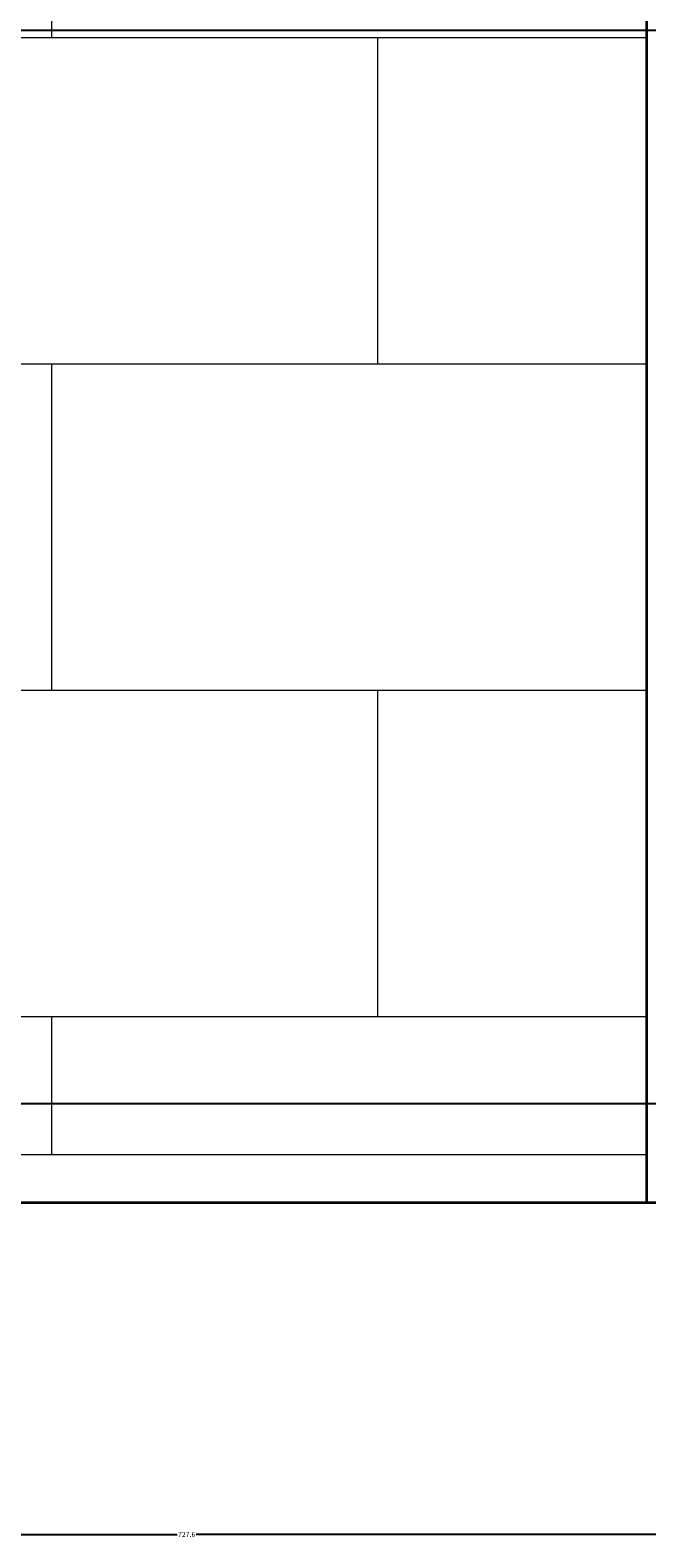
# Model space of a CAD drawing. Units: inches. Extents: x -26 to 776, y -22 to 650.
# Tile 17 of 62: x 358 to 426, y -22 to 145. Entities that reach past the tile are written whole.
import ezdxf

# ---------------------------------------------------------------- set-up
doc = ezdxf.new("R2010")
doc.units = ezdxf.units.IN
doc.header["$MEASUREMENT"] = 0
for name, color, linetype, lineweight in [('A-ANNO-DIMS', 2, 'Continuous', 18), ('A-WALL', 7, 'Continuous', 35), ('A-WALL-PATT', 8, 'Continuous', 13), ('A-WALL-TRIM', 7, 'Continuous', 18), ('C-TOPO', 7, 'Continuous', 35)]:
    doc.layers.add(name, color=color, linetype=linetype, lineweight=lineweight)
doc.styles.get("Standard").update_dxf_attribs({"font": 'arial.ttf'})
doc.dimstyles.get("Standard").update_dxf_attribs({"dimtxt": 0.5625, "dimasz": 0.18, "dimexe": 0.18, "dimexo": 0.0625, "dimgap": 0.09, "dimtad": 0, "dimtih": 1, "dimtoh": 1, "dimdec": 4, "dimzin": 0, "dimdsep": 46, "dimlunit": 4, "dimtxsty": 'Standard', "dimcen": 0.09, "dimadec": 0, "dimazin": 0, "dimtfac": 1, "dimtdec": 4, "dimtofl": 0, "dimtmove": 0, "dimatfit": 3, "dimfxl": 1, "dimtolj": 1, "dimtzin": 0, "dimarcsym": 0})

# ---------------------------------------------------------------- blocks, each defined once
blk = doc.blocks.new('*D13')
at = {"layer": 'A-ANNO-DIMS', "color": 0, "lineweight": -2, "transparency": 16777216}
for p, q in [((738.75, 50.79), (738.75, -21.31)), ((11.11, 15.42), (11.11, -21.31)), ((11.29, -21.13), (373.89, -21.13)), ((738.57, -21.13), (375.97, -21.13))]:
    blk.add_line(p, q, dxfattribs=at)
at = {"layer": 'A-ANNO-DIMS', "color": 0, "transparency": 16777216}
for points in [[(11.29, -21.1), (11.29, -21.16), (11.11, -21.13)], [(738.57, -21.1), (738.57, -21.16), (738.75, -21.13)]]:
    blk.add_solid(points, dxfattribs=at)
at = {"layer": 'Defpoints', "color": 0, "transparency": 16777216}
for p in [(738.75, 50.85), (11.11, 15.48), (738.75, -21.13)]:
    blk.add_point(p, dxfattribs=at)
at = {"layer": 'A-ANNO-DIMS', "color": 0, "transparency": 16777216, "insert": (374.93, -21.13), "char_height": 0.562, "attachment_point": 5}
blk.add_mtext('\\A1;727.6', dxfattribs=at)
blk = doc.blocks.new('*D30')
at = {"layer": 'A-ANNO-DIMS', "color": 0, "lineweight": -2, "transparency": 16777216}
for p, q in [((280.68, 144.84), (775.34, 144.84)), ((775.16, 144.66), (775.16, 86.01)), ((775.16, 26.6), (775.16, 85.25)), ((280.68, 26.42), (775.34, 26.42))]:
    blk.add_line(p, q, dxfattribs=at)
at = {"layer": 'A-ANNO-DIMS', "color": 0, "transparency": 16777216}
for points in [[(775.13, 144.66), (775.19, 144.66), (775.16, 144.84)], [(775.13, 26.6), (775.19, 26.6), (775.16, 26.42)]]:
    blk.add_solid(points, dxfattribs=at)
at = {"layer": 'Defpoints', "color": 0, "transparency": 16777216}
for p in [(280.62, 144.84), (775.16, 144.84), (280.62, 26.42)]:
    blk.add_point(p, dxfattribs=at)
at = {"layer": 'A-ANNO-DIMS', "color": 0, "transparency": 16777216, "insert": (775.16, 85.63), "char_height": 0.562, "attachment_point": 5}
blk.add_mtext('\\A1;118.41', dxfattribs=at)
blk = doc.blocks.new('*D38')
at = {"layer": 'A-ANNO-DIMS', "color": 0, "lineweight": -2, "transparency": 16777216}
for p, q in [((280.68, 26.42), (775.34, 26.42)), ((775.16, 26.24), (775.16, 21.33)), ((775.16, 15.66), (775.16, 20.58)), ((289.3, 15.48), (775.34, 15.48))]:
    blk.add_line(p, q, dxfattribs=at)
at = {"layer": 'A-ANNO-DIMS', "color": 0, "transparency": 16777216}
for points in [[(775.13, 26.24), (775.19, 26.24), (775.16, 26.42)], [(775.13, 15.66), (775.19, 15.66), (775.16, 15.48)]]:
    blk.add_solid(points, dxfattribs=at)
at = {"layer": 'Defpoints', "color": 0, "transparency": 16777216}
for p in [(280.62, 26.42), (775.16, 26.42), (289.24, 15.48)]:
    blk.add_point(p, dxfattribs=at)
at = {"layer": 'A-ANNO-DIMS', "color": 0, "transparency": 16777216, "insert": (775.16, 20.95), "char_height": 0.562, "attachment_point": 5}
blk.add_mtext('\\A1;10.942', dxfattribs=at)
blk = doc.blocks.new('*D39')
at = {"layer": 'A-ANNO-DIMS', "color": 0, "lineweight": -2, "transparency": 16777216}
for p, q in [((289.24, 15.54), (289.24, 649.86)), ((289.42, 649.68), (356.48, 649.68)), ((425.56, 649.68), (358.51, 649.68)), ((425.74, 15.54), (425.74, 649.86))]:
    blk.add_line(p, q, dxfattribs=at)
at = {"layer": 'A-ANNO-DIMS', "color": 0, "transparency": 16777216}
for points in [[(289.42, 649.71), (289.42, 649.65), (289.24, 649.68)], [(425.56, 649.71), (425.56, 649.65), (425.74, 649.68)]]:
    blk.add_solid(points, dxfattribs=at)
at = {"layer": 'Defpoints', "color": 0, "transparency": 16777216}
for p in [(425.74, 649.68), (289.24, 15.48), (425.74, 15.48)]:
    blk.add_point(p, dxfattribs=at)
at = {"layer": 'A-ANNO-DIMS', "color": 0, "transparency": 16777216, "insert": (357.49, 649.68), "char_height": 0.562, "attachment_point": 5}
blk.add_mtext('\\A1;136.5', dxfattribs=at)

msp = doc.modelspace()

# ---------------------------------------------------------------- hatches: boundary and pattern name
at = {"layer": 'A-WALL-PATT'}
h = msp.add_hatch(dxfattribs=at)
h.set_pattern_fill('AR-B816', color=256, scale=4.5)
h.paths.add_polyline_path([(425.7434, 448.2114), (289.2424, 496.9554), (289.2424, 458.1203), (289.2424, 291.1798), (289.2424, 20.7937), (425.7434, 20.7937), (425.7434, 283.2492)])

# ---------------------------------------------------------------- linework, layer by layer
at = {"layer": 'A-WALL'}
msp.add_line((425.7434, 15.4824), (425.7434, 283.2492), dxfattribs=at)
at = {"layer": 'A-WALL-TRIM'}
msp.add_line((217.9529, 20.7937), (425.7434, 20.7937), dxfattribs=at)
at = {"layer": 'C-TOPO'}
for p, q in [((289.2424, 15.4824), (425.7434, 15.4824)), ((425.7434, 15.4824), (677.9037, 15.4824))]:
    msp.add_line(p, q, dxfattribs=at)

# ---------------------------------------------------------------- dimensions: what is measured, and where the dimension line sits
at = {"layer": 'A-ANNO-DIMS'}
for base, p1, p2, picture, middle in [((425.7434, 649.6763), (289.2424, 15.4824), (425.7434, 15.4824), '*D39', (357.4929, 649.6763)), ((738.7503, -21.1349), (11.1074, 15.4824), (738.7503, 50.8482), '*D13', (374.9289, -21.1349))]:
    dim = msp.add_linear_dim(base=base, p1=p1, p2=p2, dimstyle='Standard', override={"dimdec": 1, "dimlfac": 1, "dimrnd": 0, "dimzin": 0, "dimdsep": 46, "dimlunit": 2}, dxfattribs=at)
    dim.commit()
    dim.dimension.update_dxf_attribs({"geometry": picture, "text_midpoint": middle})
for base, p1, p2, override, picture, middle in [((775.1553, 144.8359), (280.6173, 26.4239), (280.6173, 144.8359), {"dimdec": 2, "dimlfac": 1, "dimrnd": 0, "dimzin": 0, "dimdsep": 46, "dimlunit": 2}, '*D30', (775.1553, 85.6299)), ((775.15535, 26.4239), (289.24236, 15.48237), (280.61732, 26.4239), {"dimdec": 3, "dimlfac": 1, "dimrnd": 0, "dimzin": 0, "dimdsep": 46, "dimlunit": 2}, '*D38', (775.15535, 20.95313))]:
    dim = msp.add_linear_dim(base=base, p1=p1, p2=p2, angle=90, dimstyle='Standard', override=override, dxfattribs=at)
    dim.commit()
    dim.dimension.update_dxf_attribs({"geometry": picture, "text_midpoint": middle})

doc.saveas('drawing.dxf')
